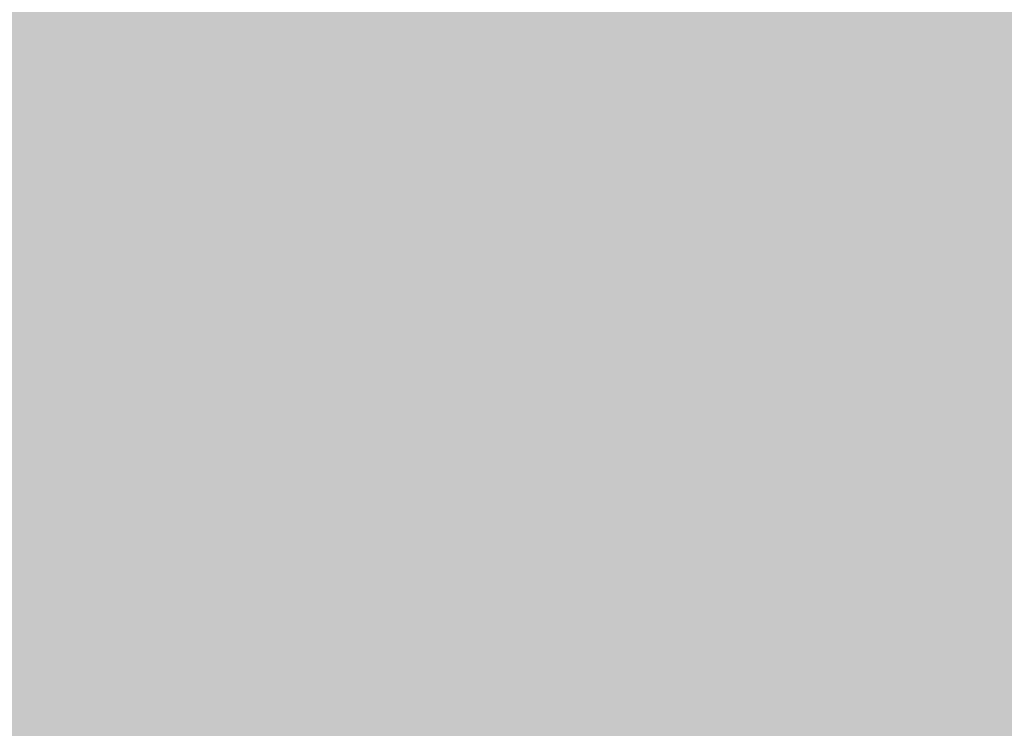
# Model space of a CAD drawing. Units: feet. Extents: x 3168 to 4724, y 827 to 1477.
# Tile 131 of 256: x 3300.858 to 3303.032, y 1096.781 to 1098.344. Entities that reach past the tile are written whole.
import ezdxf

# ---------------------------------------------------------------- set-up
doc = ezdxf.new("R2010")
doc.units = ezdxf.units.FT
doc.layers.add('A-ELEV-PATT', color=8, linetype='Continuous', lineweight=13)

msp = doc.modelspace()

# ---------------------------------------------------------------- hatches: boundary and pattern name
at = {"layer": 'A-ELEV-PATT'}
h = msp.add_hatch(color=256, dxfattribs=at)
h.dxf.hatch_style = 1
edge = h.paths.add_edge_path()
edge.add_ellipse((3552.9058, 979.2201), major_axis=(36.7449, 0), ratio=0.4848485, start_angle=0, end_angle=360)
edge = h.paths.add_edge_path()
edge.add_ellipse((3559.8916, 929.2523), major_axis=(36.7449, 0), ratio=0.4848485, start_angle=0, end_angle=360)
edge = h.paths.add_edge_path()
edge.add_line((3299.3168, 1198.6061), (3479.9167, 1198.6061))
edge.add_line((3479.9167, 1198.6061), (3479.9167, 1209.8686))
edge.add_spline(control_points=[(3479.9167, 1209.8686), (3464.3012, 1209.8686), (3448.6856, 1209.8686), (3410.9491, 1209.8686), (3388.8282, 1209.8686), (3355.6469, 1209.8686), (3344.5864, 1209.8686), (3327.9957, 1209.8686), (3322.4655, 1209.8686), (3314.1702, 1209.8686), (3311.4051, 1209.8686), (3307.2574, 1209.8686), (3305.8748, 1209.8686), (3303.801, 1209.8686), (3303.1097, 1209.8686), (3302.0728, 1209.8686), (3301.7272, 1209.8686), (3301.2087, 1209.8686), (3301.0359, 1209.8686), (3300.7767, 1209.8686), (3300.6903, 1209.8686), (3300.5606, 1209.8686), (3300.5174, 1209.8686), (3300.4526, 1209.8686), (3300.431, 1209.8686), (3300.3986, 1209.8686), (3300.3878, 1209.8686), (3300.3662, 1209.8686), (3300.3457, 1209.8686), (3300.3455, 1209.8686), (3300.3455, 1209.8686), (3300.3433, 1209.8686), (3300.3411, 1209.8686), (3300.3379, 1209.8686), (3300.3368, 1209.8686), (3300.3339, 1209.8686), (3300.3321, 1209.8686), (3300.3255, 1209.8686), (3300.3207, 1209.8686), (3300.3109, 1209.8686), (3300.306, 1209.8686), (3300.2905, 1209.8686), (3300.28, 1209.8686), (3300.2324, 1209.8688), (3300.1953, 1209.869), (3299.9511, 1209.8706), (3299.7448, 1209.8743), (3299.4368, 1209.8833), (3299.3344, 1209.8868), (3299.1811, 1209.8929), (3299.13, 1209.8951), (3298.6522, 1209.9168), (3298.2295, 1209.9457), (3297.6016, 1210.0024), (3297.3934, 1210.0235), (3297.0827, 1210.0583), (3296.9793, 1210.0705), (3296.293, 1210.1549), (3295.7181, 1210.2434), (3294.8687, 1210.3989), (3294.5877, 1210.4545), (3294.1693, 1210.5433), (3294.0304, 1210.5739), (3291.7071, 1211.1012), (3289.6536, 1211.8134), (3285.7763, 1213.564), (3283.9514, 1214.6035), (3280.5122, 1216.9801), (3278.8972, 1218.3176), (3276.3799, 1220.8295), (3275.416, 1221.9177), (3274.0393, 1223.7077), (3273.581, 1224.3495), (3273.1432, 1225.0163)], knot_values=[39.119033, 39.119033, 39.119033, 39.119033, 39.286353, 39.286353, 39.523379, 39.523379, 39.641892, 39.641892, 39.701148, 39.701148, 39.730777, 39.730777, 39.745591, 39.745591, 39.752998, 39.752998, 39.756701, 39.756701, 39.758553, 39.758553, 39.759479, 39.759479, 39.759942, 39.759942, 39.760173, 39.760173, 39.760289, 39.760289, 39.760405, 39.760405, 39.760463, 39.760463, 39.763389, 39.763389, 39.764851, 39.764851, 39.767304, 39.767304, 39.773825, 39.773825, 39.78057, 39.78057, 39.79477, 39.79477, 39.845194, 39.845194, 40.126715, 40.126715, 40.267476, 40.267476, 40.337856, 40.337856, 40.927023, 40.927023, 41.221606, 41.221606, 41.368898, 41.368898, 42.202622, 42.202622, 42.619485, 42.619485, 42.827916, 42.827916, 46.118323, 46.118323, 49.408731, 49.408731, 52.699139, 52.699139, 54.927489, 54.927489, 56.104228, 56.104228, 56.104228, 56.104228], weights=[1, 1, 1, 1, 1, 1, 1, 1, 1, 1, 1, 1, 1, 1, 1, 1, 1, 1, 1, 1, 1, 1, 1, 1, 1, 1, 1, 1, 1, 1, 1, 1, 1, 1, 1, 1, 1, 1, 1, 1, 1, 1, 1, 1, 1, 1, 1, 1, 1, 1, 1, 1, 1, 1, 1, 1, 1, 1, 1, 1, 1, 1, 1, 1, 1, 1, 1, 1, 1, 1, 1, 1, 1, 1], degree=3, periodic=0)
edge.add_line((3273.1432, 1225.0163), (3273.1432, 1099.0163))
edge.add_line((3273.1432, 1099.0163), (3299.3168, 1099.0163))
edge.add_line((3299.3168, 1099.0163), (3299.3168, 1198.6061))
edge = h.paths.add_edge_path()
edge.add_line((3304.7584, 1324.1581), (3479.9167, 1324.1581))
edge.add_line((3479.9167, 1324.1581), (3479.9167, 1335.7146))
edge.add_line((3479.9167, 1335.7146), (3269.1616, 1335.7146))
edge.add_spline(control_points=[(3269.1616, 1335.7146), (3264.0242, 1335.7146), (3258.3641, 1328.9582), (3259.2643, 1323.9003)], knot_values=[0, 0, 0, 0, 15.412191, 15.412191, 15.412191, 15.412191], degree=3, periodic=0)
edge.add_line((3259.2643, 1323.9003), (3265.5168, 1288.7691))
edge.add_line((3265.5168, 1288.7691), (3275.2651, 1261.5456))
edge.add_line((3275.2651, 1261.5456), (3304.7584, 1261.5456))
edge.add_line((3304.7584, 1261.5456), (3304.7584, 1324.1581))
h = msp.add_hatch(color=256, dxfattribs=at)
h.dxf.hatch_style = 1
h.paths.add_polyline_path([(3384.5252, 1099.0163), (3335.0292, 1099.0163), (3299.3168, 1099.0163), (3273.1432, 1099.0163), (3217.5654, 1099.0163), (3168.0693, 827.1163), (3335.0292, 827.1163)])

doc.saveas('drawing.dxf')
